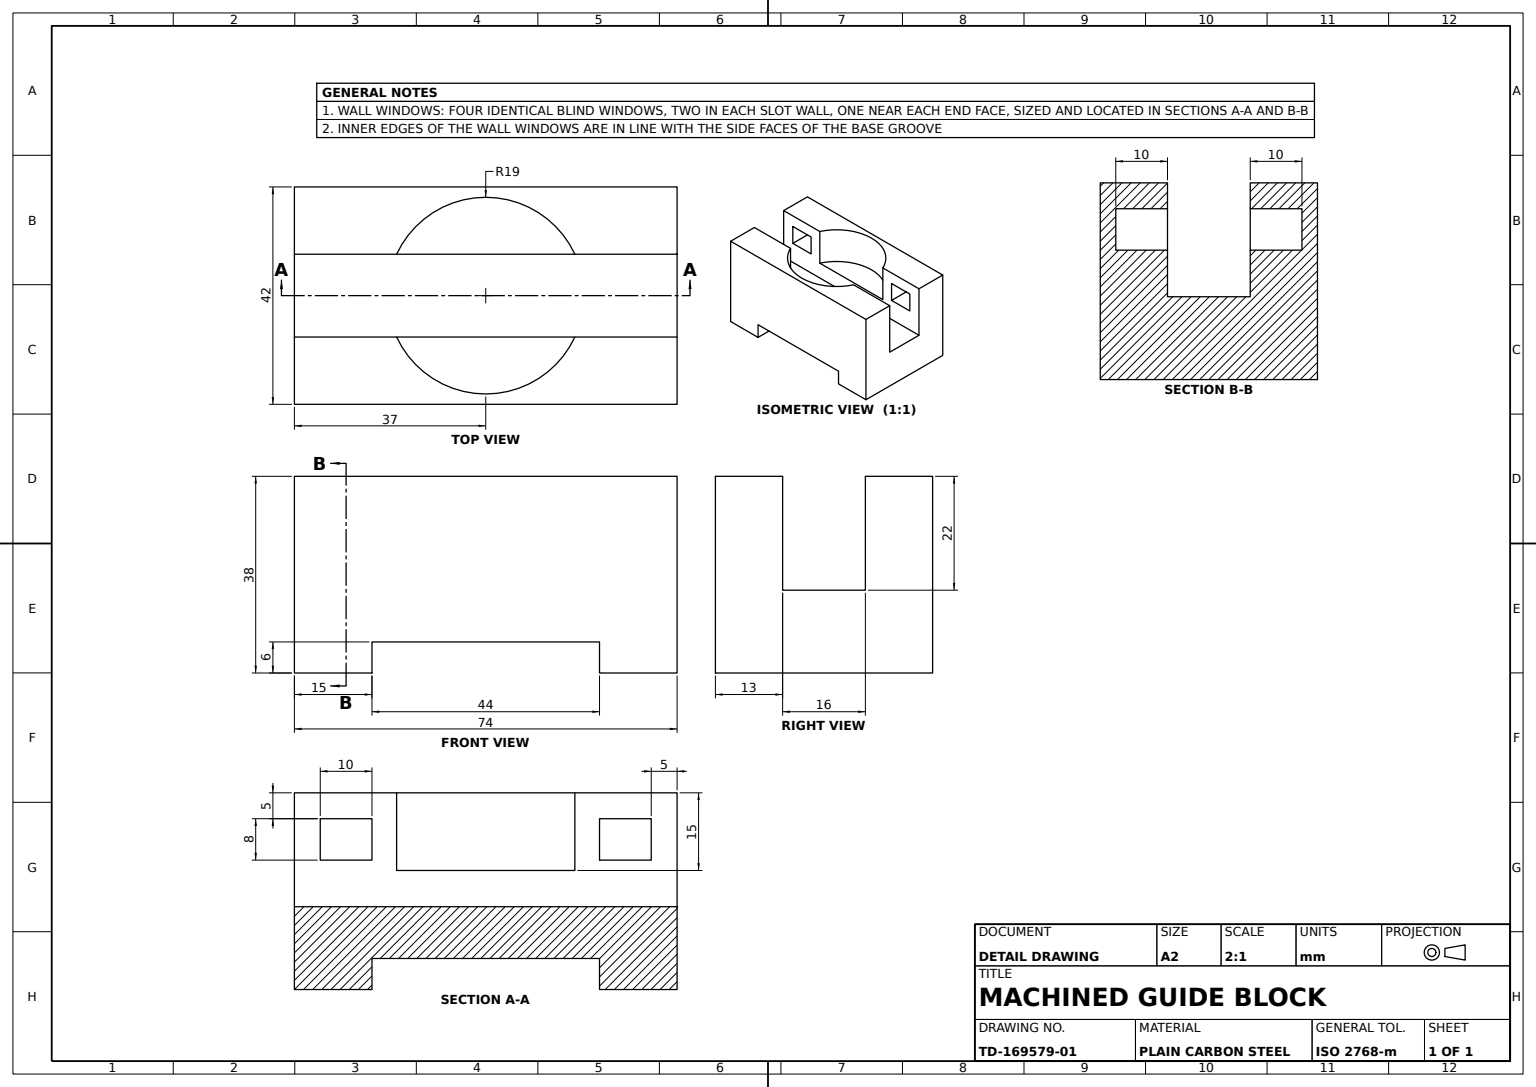
from build123d import *

# Parameters (mm, degrees)
BLOCK_BODY_DEPTH          = 74
BASE_GROOVE_SKETCH_W      = 44
BASE_GROOVE_SKETCH_H      = 6
BASE_GROOVE_44X6_DEPTH    = 94.187982058
BORE_SKETCH_R             = 19
BORE_38_DEPTH             = 15
WALL_WINDOWS_A_SKETCH_W   = 10
WALL_WINDOWS_A_SKETCH_H   = 8
WALL_WINDOWS_A_10X8_DEPTH = 10
WALL_WINDOWS_B_SKETCH_W   = 10
WALL_WINDOWS_B_SKETCH_H   = 8
WALL_WINDOWS_B_10X8_DEPTH = 10


with BuildPart() as part:
    # Block Profile Sketch → Block Body (new body)
    with BuildSketch(Plane.XY):
        Polygon((-21, 0), (21, 0), (21, 38), (8, 38), (8, 16), (-8, 16), (-8, 38), (-21, 38), align=None)
    extrude(amount=-BLOCK_BODY_DEPTH)

    # Base Groove Sketch → Base Groove 44x6 (cut, through all)
    with BuildSketch(Plane(origin=(21, 0, 0), x_dir=(0, 0, -1), z_dir=(1, 0, 0))):
        with Locations((37, 3)):
            Rectangle(BASE_GROOVE_SKETCH_W, BASE_GROOVE_SKETCH_H)
    extrude(amount=-BASE_GROOVE_44X6_DEPTH, mode=Mode.SUBTRACT)

    # Bore Sketch → Bore Ø38 (cut)
    with BuildSketch(Plane(origin=(0, 38, 0), x_dir=(1, 0, 0), z_dir=(0, 1, 0))):
        with Locations((0, 37)):
            Circle(BORE_SKETCH_R)
    extrude(amount=-BORE_38_DEPTH, mode=Mode.SUBTRACT)

    # Wall Windows A Sketch → Wall Windows A 10x8 (cut)
    with BuildSketch(Plane(origin=(-8, 0, 0), x_dir=(0, 0, -1), z_dir=(1, 0, 0))):
        with Locations((10, 29)):
            Rectangle(WALL_WINDOWS_A_SKETCH_W, WALL_WINDOWS_A_SKETCH_H)
        with Locations((64, 29)):
            Rectangle(WALL_WINDOWS_A_SKETCH_W, WALL_WINDOWS_A_SKETCH_H)
    extrude(amount=-WALL_WINDOWS_A_10X8_DEPTH, mode=Mode.SUBTRACT)

    # Wall Windows B Sketch → Wall Windows B 10x8 (cut)
    with BuildSketch(Plane.ZY.offset(-8)):
        with Locations((-64, 29)):
            Rectangle(WALL_WINDOWS_B_SKETCH_W, WALL_WINDOWS_B_SKETCH_H)
        with Locations((-10, 29)):
            Rectangle(WALL_WINDOWS_B_SKETCH_W, WALL_WINDOWS_B_SKETCH_H)
    extrude(amount=-WALL_WINDOWS_B_10X8_DEPTH, mode=Mode.SUBTRACT)


solid = part.part
